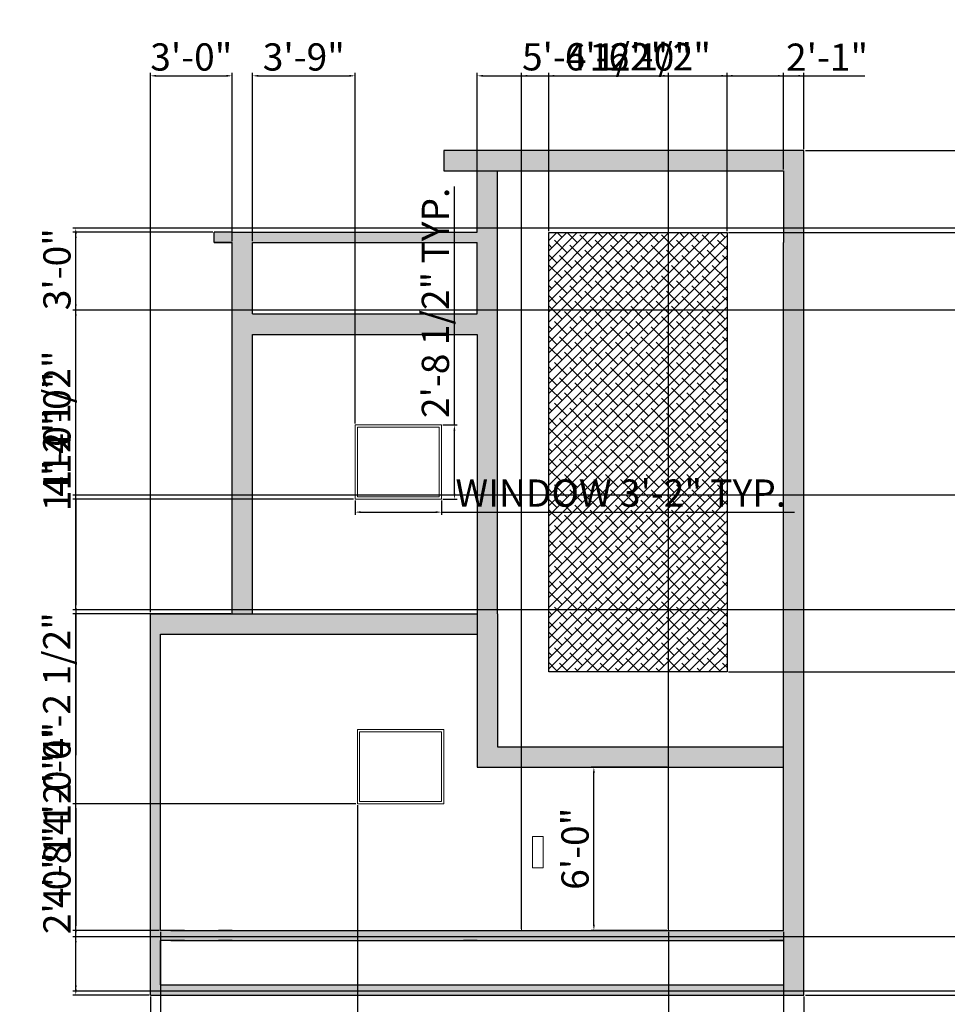
# Model space of a CAD drawing. Units: inches. Extents: x 2693 to 3501, y 1190 to 2292.
# Tile 3 of 4: x 2693 to 3102, y 1858 to 2292. Entities that reach past the tile are written whole.
import ezdxf

# ---------------------------------------------------------------- set-up
doc = ezdxf.new("R2010")
doc.units = ezdxf.units.IN
for name, color, linetype, lineweight in [('A-ANNO-DIMS', 2, 'Continuous', 18), ('A-DOOR', 3, 'Continuous', 18), ('A-ELEV', 7, 'Continuous', 25), ('A-ELEV-PATT', 252, 'Continuous', 13), ('A-GLAZ', 4, 'Continuous', 18), ('A-SECT-PATT', 252, 'Continuous', 13)]:
    doc.layers.add(name, color=color, linetype=linetype, lineweight=lineweight)
doc.styles.get("Standard").update_dxf_attribs({"font": 'arial.ttf'})
doc.dimstyles.new('ISO-25', dxfattribs={"dimtxt": 12, "dimasz": 2.5, "dimexe": 1.25, "dimexo": 0.625, "dimtad": 1, "dimdec": 1, "dimlunit": 3, "dimtxsty": 'Standard', "dimcen": 2.5, "dimadec": 0, "dimazin": 0, "dimtfac": 1, "dimtdec": 1, "dimtmove": 0, "dimatfit": 3, "dimfxl": 1, "dimarcsym": 0})

# ---------------------------------------------------------------- blocks, each defined once
blk = doc.blocks.new('WIN-ELEV-RECT-38')
for points in [[(0, 32.69), (38.06, 32.69), (38.06, 0), (0, 0)], [(1, 31.69), (37.06, 31.69), (37.06, 1), (1, 1)]]:
    blk.add_lwpolyline(points, close=True)
blk = doc.blocks.new('*D15')
at = {"layer": 'A-ANNO-DIMS', "color": 0, "lineweight": -2, "transparency": 16777216}
for p, q in [((2840.85, 2079.8), (2840.85, 2073.46)), ((2878.91, 2079.8), (2878.91, 2073.46)), ((2843.35, 2074.71), (2876.41, 2074.71)), ((2878.91, 2074.71), (3034.51, 2074.71))]:
    blk.add_line(p, q, dxfattribs=at)
at = {"layer": 'A-ANNO-DIMS', "color": 0, "transparency": 16777216}
for points in [[(2843.35, 2075.13), (2843.35, 2074.3), (2840.85, 2074.71)], [(2876.41, 2075.13), (2876.41, 2074.3), (2878.91, 2074.71)]]:
    blk.add_solid(points, dxfattribs=at)
at = {"layer": 'Defpoints', "color": 0, "transparency": 16777216}
for p in [(2840.85, 2080.42), (2878.91, 2080.42), (2878.91, 2074.71)]:
    blk.add_point(p, dxfattribs=at)
at = {"layer": 'A-ANNO-DIMS', "color": 0, "transparency": 16777216, "insert": (2957.96, 2081.55), "char_height": 12, "attachment_point": 5}
blk.add_mtext('WINDOW 3\'-2" TYP.', dxfattribs=at)
blk = doc.blocks.new('*D16')
at = {"layer": 'A-ANNO-DIMS', "color": 0, "lineweight": -2, "transparency": 16777216}
for p, q in [((2884.62, 2113.11), (2884.62, 2218.17)), ((2879.54, 2113.11), (2885.87, 2113.11)), ((2884.62, 2082.92), (2884.62, 2110.61)), ((2879.54, 2080.42), (2885.87, 2080.42))]:
    blk.add_line(p, q, dxfattribs=at)
at = {"layer": 'A-ANNO-DIMS', "color": 0, "transparency": 16777216}
for points in [[(2884.21, 2110.61), (2885.04, 2110.61), (2884.62, 2113.11)], [(2884.21, 2082.92), (2885.04, 2082.92), (2884.62, 2080.42)]]:
    blk.add_solid(points, dxfattribs=at)
at = {"layer": 'Defpoints', "color": 0, "transparency": 16777216}
for p in [(2878.91, 2113.11), (2884.62, 2113.11), (2878.91, 2080.42)]:
    blk.add_point(p, dxfattribs=at)
at = {"layer": 'A-ANNO-DIMS', "color": 0, "transparency": 16777216, "insert": (2877.79, 2166.89), "char_height": 12, "attachment_point": 5, "rotation": 90}
blk.add_mtext('2\'-8 1/2" TYP.', dxfattribs=at)
blk = doc.blocks.new('*D32')
at = {"layer": 'A-ANNO-DIMS', "color": 0, "lineweight": -2, "transparency": 16777216}
for p, q in [((2750.68, 2030.62), (2750.68, 2268.14)), ((2753.18, 2266.89), (2784.18, 2266.89)), ((2786.68, 2194.12), (2786.68, 2268.14))]:
    blk.add_line(p, q, dxfattribs=at)
at = {"layer": 'A-ANNO-DIMS', "color": 0, "transparency": 16777216}
for points in [[(2753.18, 2267.31), (2753.18, 2266.48), (2750.68, 2266.89)], [(2784.18, 2267.31), (2784.18, 2266.48), (2786.68, 2266.89)]]:
    blk.add_solid(points, dxfattribs=at)
at = {"layer": 'Defpoints', "color": 0, "transparency": 16777216}
for p in [(2786.68, 2266.89), (2786.68, 2193.49), (2750.68, 2029.99)]:
    blk.add_point(p, dxfattribs=at)
at = {"layer": 'A-ANNO-DIMS', "color": 0, "transparency": 16777216, "insert": (2768.68, 2273.65), "char_height": 12, "attachment_point": 5}
blk.add_mtext('3\'-0"', dxfattribs=at)
blk = doc.blocks.new('*D33')
at = {"layer": 'A-ANNO-DIMS', "color": 0, "lineweight": -2, "transparency": 16777216}
for p, q in [((2894.68, 2198.62), (2894.68, 2268.14)), ((2897.18, 2266.89), (3036.18, 2266.89)), ((3038.68, 2234.62), (3038.68, 2268.14))]:
    blk.add_line(p, q, dxfattribs=at)
at = {"layer": 'A-ANNO-DIMS', "color": 0, "transparency": 16777216}
for points in [[(2897.18, 2267.31), (2897.18, 2266.48), (2894.68, 2266.89)], [(3036.18, 2267.31), (3036.18, 2266.48), (3038.68, 2266.89)]]:
    blk.add_solid(points, dxfattribs=at)
at = {"layer": 'Defpoints', "color": 0, "transparency": 16777216}
for p in [(3038.68, 2266.89), (3038.68, 2233.99), (2894.68, 2197.99)]:
    blk.add_point(p, dxfattribs=at)
at = {"layer": 'A-ANNO-DIMS', "color": 0, "transparency": 16777216, "insert": (2966.68, 2273.65), "char_height": 12, "attachment_point": 5}
blk.add_mtext('12\'-0"', dxfattribs=at)
blk = doc.blocks.new('*D34')
at = {"layer": 'A-ANNO-DIMS', "color": 0, "lineweight": -2, "transparency": 16777216}
for p, q in [((2750.05, 2029.99), (2716.53, 2029.99)), ((2717.78, 1864.49), (2717.78, 2027.49)), ((2750.05, 1861.99), (2716.53, 1861.99))]:
    blk.add_line(p, q, dxfattribs=at)
at = {"layer": 'A-ANNO-DIMS', "color": 0, "transparency": 16777216}
for points in [[(2717.36, 2027.49), (2718.19, 2027.49), (2717.78, 2029.99)], [(2717.36, 1864.49), (2718.19, 1864.49), (2717.78, 1861.99)]]:
    blk.add_solid(points, dxfattribs=at)
at = {"layer": 'Defpoints', "color": 0, "transparency": 16777216}
for p in [(2717.78, 2029.99), (2750.68, 2029.99), (2750.68, 1861.99)]:
    blk.add_point(p, dxfattribs=at)
at = {"layer": 'A-ANNO-DIMS', "color": 0, "transparency": 16777216, "insert": (2711.02, 1945.99), "char_height": 12, "attachment_point": 5, "rotation": 90}
blk.add_mtext('14\'-0"', dxfattribs=at)
blk = doc.blocks.new('*D35')
at = {"layer": 'A-ANNO-DIMS', "color": 0, "lineweight": -2, "transparency": 16777216}
for p, q in [((2778.13, 2197.99), (2716.53, 2197.99)), ((2717.78, 2032.49), (2717.78, 2195.49)), ((2786.05, 2029.99), (2716.53, 2029.99))]:
    blk.add_line(p, q, dxfattribs=at)
at = {"layer": 'A-ANNO-DIMS', "color": 0, "transparency": 16777216}
for points in [[(2717.36, 2195.49), (2718.19, 2195.49), (2717.78, 2197.99)], [(2717.36, 2032.49), (2718.19, 2032.49), (2717.78, 2029.99)]]:
    blk.add_solid(points, dxfattribs=at)
at = {"layer": 'Defpoints', "color": 0, "transparency": 16777216}
for p in [(2717.78, 2197.99), (2778.76, 2197.99), (2786.68, 2029.99)]:
    blk.add_point(p, dxfattribs=at)
at = {"layer": 'A-ANNO-DIMS', "color": 0, "transparency": 16777216, "insert": (2711.02, 2113.99), "char_height": 12, "attachment_point": 5, "rotation": 90}
blk.add_mtext('14\'-0"', dxfattribs=at)
blk = doc.blocks.new('*D36')
at = {"layer": 'A-ANNO-DIMS', "color": 0, "lineweight": -2, "transparency": 16777216}
for p, q in [((2841.85, 1945.66), (2841.85, 1804.29)), ((2755.18, 1889.87), (2755.18, 1804.29)), ((2757.68, 1805.54), (2839.35, 1805.54))]:
    blk.add_line(p, q, dxfattribs=at)
at = {"layer": 'A-ANNO-DIMS', "color": 0, "transparency": 16777216}
for points in [[(2757.68, 1805.95), (2757.68, 1805.12), (2755.18, 1805.54)], [(2839.35, 1805.95), (2839.35, 1805.12), (2841.85, 1805.54)]]:
    blk.add_solid(points, dxfattribs=at)
at = {"layer": 'Defpoints', "color": 0, "transparency": 16777216}
for p in [(2841.85, 1946.28), (2755.18, 1890.49), (2841.85, 1805.54)]:
    blk.add_point(p, dxfattribs=at)
at = {"layer": 'A-ANNO-DIMS', "color": 0, "transparency": 16777216, "insert": (2798.51, 1812.37), "char_height": 12, "attachment_point": 5}
blk.add_mtext('7\'-2 1/2"', dxfattribs=at)
blk = doc.blocks.new('*D37')
at = {"layer": 'A-ANNO-DIMS', "color": 0, "lineweight": -2, "transparency": 16777216}
for p, q in [((2841.23, 1946.28), (2716.53, 1946.28)), ((2717.78, 1943.78), (2717.78, 1892.99)), ((2754.55, 1890.49), (2716.53, 1890.49))]:
    blk.add_line(p, q, dxfattribs=at)
at = {"layer": 'A-ANNO-DIMS', "color": 0, "transparency": 16777216}
for points in [[(2717.36, 1943.78), (2718.19, 1943.78), (2717.78, 1946.28)], [(2717.36, 1892.99), (2718.19, 1892.99), (2717.78, 1890.49)]]:
    blk.add_solid(points, dxfattribs=at)
at = {"layer": 'Defpoints', "color": 0, "transparency": 16777216}
for p in [(2841.85, 1946.28), (2717.78, 1890.49), (2755.18, 1890.49)]:
    blk.add_point(p, dxfattribs=at)
at = {"layer": 'A-ANNO-DIMS', "color": 0, "transparency": 16777216, "insert": (2711.02, 1918.39), "char_height": 12, "attachment_point": 5, "rotation": 90}
blk.add_mtext('4\'-8"', dxfattribs=at)
blk = doc.blocks.new('*D38')
at = {"layer": 'A-ANNO-DIMS', "color": 0, "lineweight": -2, "transparency": 16777216}
for p, q in [((2717.78, 2080.42), (2717.78, 2144.52)), ((2840.23, 2080.42), (2716.53, 2080.42)), ((2717.78, 2032.49), (2717.78, 2077.92)), ((2786.05, 2029.99), (2716.53, 2029.99))]:
    blk.add_line(p, q, dxfattribs=at)
at = {"layer": 'A-ANNO-DIMS', "color": 0, "transparency": 16777216}
for points in [[(2717.36, 2077.92), (2718.19, 2077.92), (2717.78, 2080.42)], [(2717.36, 2032.49), (2718.19, 2032.49), (2717.78, 2029.99)]]:
    blk.add_solid(points, dxfattribs=at)
at = {"layer": 'Defpoints', "color": 0, "transparency": 16777216}
for p in [(2717.78, 2080.42), (2840.85, 2080.42), (2786.68, 2029.99)]:
    blk.add_point(p, dxfattribs=at)
at = {"layer": 'A-ANNO-DIMS', "color": 0, "transparency": 16777216, "insert": (2710.95, 2113.72), "char_height": 12, "attachment_point": 5, "rotation": 90}
blk.add_mtext('4\'-2 1/2"', dxfattribs=at)
blk = doc.blocks.new('*D39')
at = {"layer": 'A-ANNO-DIMS', "color": 0, "lineweight": -2, "transparency": 16777216}
for p, q in [((2795.68, 2194.12), (2795.68, 2268.14)), ((2798.18, 2266.89), (2838.35, 2266.89)), ((2840.85, 2113.74), (2840.85, 2268.14))]:
    blk.add_line(p, q, dxfattribs=at)
at = {"layer": 'A-ANNO-DIMS', "color": 0, "transparency": 16777216}
for points in [[(2798.18, 2267.31), (2798.18, 2266.48), (2795.68, 2266.89)], [(2838.35, 2267.31), (2838.35, 2266.48), (2840.85, 2266.89)]]:
    blk.add_solid(points, dxfattribs=at)
at = {"layer": 'Defpoints', "color": 0, "transparency": 16777216}
for p in [(2840.85, 2266.89), (2795.68, 2193.49), (2840.85, 2113.11)]:
    blk.add_point(p, dxfattribs=at)
at = {"layer": 'A-ANNO-DIMS', "color": 0, "transparency": 16777216, "insert": (2818.26, 2273.65), "char_height": 12, "attachment_point": 5}
blk.add_mtext('3\'-9"', dxfattribs=at)
blk = doc.blocks.new('*D40')
at = {"layer": 'A-ANNO-DIMS', "color": 0, "lineweight": -2, "transparency": 16777216}
for p, q in [((2914.25, 1891.12), (2914.25, 2268.14)), ((2916.75, 2266.89), (2976.49, 2266.89)), ((2978.99, 1891.12), (2978.99, 2268.14))]:
    blk.add_line(p, q, dxfattribs=at)
at = {"layer": 'A-ANNO-DIMS', "color": 0, "transparency": 16777216}
for points in [[(2916.75, 2267.31), (2916.75, 2266.48), (2914.25, 2266.89)], [(2976.49, 2267.31), (2976.49, 2266.48), (2978.99, 2266.89)]]:
    blk.add_solid(points, dxfattribs=at)
at = {"layer": 'Defpoints', "color": 0, "transparency": 16777216}
for p in [(2978.99, 2266.89), (2914.25, 1890.49), (2978.99, 1890.49)]:
    blk.add_point(p, dxfattribs=at)
at = {"layer": 'A-ANNO-DIMS', "color": 0, "transparency": 16777216, "insert": (2946.62, 2273.72), "char_height": 12, "attachment_point": 5}
blk.add_mtext('5\'-4 1/2"', dxfattribs=at)
blk = doc.blocks.new('*D41')
at = {"layer": 'A-ANNO-DIMS', "color": 0, "lineweight": -2, "transparency": 16777216}
for p, q in [((2978.99, 1889.87), (2978.99, 1804.29)), ((3029.68, 1889.87), (3029.68, 1804.29)), ((2981.49, 1805.54), (3027.18, 1805.54)), ((3029.68, 1805.54), (3093.77, 1805.54))]:
    blk.add_line(p, q, dxfattribs=at)
at = {"layer": 'A-ANNO-DIMS', "color": 0, "transparency": 16777216}
for points in [[(2981.49, 1805.95), (2981.49, 1805.12), (2978.99, 1805.54)], [(3027.18, 1805.95), (3027.18, 1805.12), (3029.68, 1805.54)]]:
    blk.add_solid(points, dxfattribs=at)
at = {"layer": 'Defpoints', "color": 0, "transparency": 16777216}
for p in [(2978.99, 1890.49), (3029.68, 1890.49), (3029.68, 1805.54)]:
    blk.add_point(p, dxfattribs=at)
at = {"layer": 'A-ANNO-DIMS', "color": 0, "transparency": 16777216, "insert": (3062.97, 1812.37), "char_height": 12, "attachment_point": 5}
blk.add_mtext('4\'-2 1/2"', dxfattribs=at)
blk = doc.blocks.new('*D42')
at = {"layer": 'A-ANNO-DIMS', "color": 0, "lineweight": -2, "transparency": 16777216}
for p, q in [((2978.36, 1962.38), (2944.84, 1962.38)), ((2946.09, 1892.99), (2946.09, 1959.88)), ((2978.36, 1890.49), (2944.84, 1890.49))]:
    blk.add_line(p, q, dxfattribs=at)
at = {"layer": 'A-ANNO-DIMS', "color": 0, "transparency": 16777216}
for points in [[(2945.67, 1959.88), (2946.5, 1959.88), (2946.09, 1962.38)], [(2945.67, 1892.99), (2946.5, 1892.99), (2946.09, 1890.49)]]:
    blk.add_solid(points, dxfattribs=at)
at = {"layer": 'Defpoints', "color": 0, "transparency": 16777216}
for p in [(2946.09, 1962.38), (2978.99, 1962.38), (2978.99, 1890.49)]:
    blk.add_point(p, dxfattribs=at)
at = {"layer": 'A-ANNO-DIMS', "color": 0, "transparency": 16777216, "insert": (2939.33, 1926.44), "char_height": 12, "attachment_point": 5, "rotation": 90}
blk.add_mtext('6\'-0"', dxfattribs=at)
blk = doc.blocks.new('*D43')
at = {"layer": 'A-ANNO-DIMS', "color": 0, "lineweight": -2, "transparency": 16777216}
for p, q in [((2926.19, 2198.48), (2926.19, 2268.14)), ((2928.69, 2266.89), (3002.26, 2266.89)), ((3004.76, 2198.48), (3004.76, 2268.14))]:
    blk.add_line(p, q, dxfattribs=at)
at = {"layer": 'A-ANNO-DIMS', "color": 0, "transparency": 16777216}
for points in [[(2928.69, 2267.31), (2928.69, 2266.48), (2926.19, 2266.89)], [(3002.26, 2267.31), (3002.26, 2266.48), (3004.76, 2266.89)]]:
    blk.add_solid(points, dxfattribs=at)
at = {"layer": 'Defpoints', "color": 0, "transparency": 16777216}
for p in [(3004.76, 2266.89), (2926.19, 2197.86), (3004.76, 2197.86)]:
    blk.add_point(p, dxfattribs=at)
at = {"layer": 'A-ANNO-DIMS', "color": 0, "transparency": 16777216, "insert": (2965.47, 2273.72), "char_height": 12, "attachment_point": 5}
blk.add_mtext('6\'-6 1/2"', dxfattribs=at)
blk = doc.blocks.new('*D44')
at = {"layer": 'A-ANNO-DIMS', "color": 0, "lineweight": -2, "transparency": 16777216}
for p, q in [((3004.76, 2198.48), (3004.76, 2268.14)), ((3007.26, 2266.89), (3027.18, 2266.89)), ((3029.68, 2225.62), (3029.68, 2268.14)), ((3029.68, 2266.89), (3065.53, 2266.89))]:
    blk.add_line(p, q, dxfattribs=at)
at = {"layer": 'A-ANNO-DIMS', "color": 0, "transparency": 16777216}
for points in [[(3007.26, 2267.31), (3007.26, 2266.48), (3004.76, 2266.89)], [(3027.18, 2267.31), (3027.18, 2266.48), (3029.68, 2266.89)]]:
    blk.add_solid(points, dxfattribs=at)
at = {"layer": 'Defpoints', "color": 0, "transparency": 16777216}
for p in [(3029.68, 2266.89), (3029.68, 2224.99), (3004.76, 2197.86)]:
    blk.add_point(p, dxfattribs=at)
at = {"layer": 'A-ANNO-DIMS', "color": 0, "transparency": 16777216, "insert": (3048.85, 2273.54), "char_height": 12, "attachment_point": 5}
blk.add_mtext('2\'-1"', dxfattribs=at)
blk = doc.blocks.new('*D45')
at = {"layer": 'A-ANNO-DIMS', "color": 0, "lineweight": -2, "transparency": 16777216}
for p, q in [((3005.39, 2197.86), (3435.42, 2197.86)), ((3434.17, 2006.84), (3434.17, 2195.36)), ((3005.39, 2004.34), (3435.42, 2004.34))]:
    blk.add_line(p, q, dxfattribs=at)
at = {"layer": 'A-ANNO-DIMS', "color": 0, "transparency": 16777216}
for points in [[(3433.76, 2195.36), (3434.59, 2195.36), (3434.17, 2197.86)], [(3433.76, 2006.84), (3434.59, 2006.84), (3434.17, 2004.34)]]:
    blk.add_solid(points, dxfattribs=at)
at = {"layer": 'Defpoints', "color": 0, "transparency": 16777216}
for p in [(3004.76, 2197.86), (3434.17, 2197.86), (3004.76, 2004.34)]:
    blk.add_point(p, dxfattribs=at)
at = {"layer": 'A-ANNO-DIMS', "color": 0, "transparency": 16777216, "insert": (3427.34, 2101.1), "char_height": 12, "attachment_point": 5, "rotation": 90}
blk.add_mtext('16\'-1 1/2"', dxfattribs=at)
blk = doc.blocks.new('*D46')
at = {"layer": 'A-ANNO-DIMS', "color": 0, "lineweight": -2, "transparency": 16777216}
for p, q in [((2750.68, 1861.37), (2750.68, 1804.29)), ((3038.68, 1861.37), (3038.68, 1804.29)), ((2753.18, 1805.54), (3036.18, 1805.54))]:
    blk.add_line(p, q, dxfattribs=at)
at = {"layer": 'A-ANNO-DIMS', "color": 0, "transparency": 16777216}
for points in [[(2753.18, 1805.95), (2753.18, 1805.12), (2750.68, 1805.54)], [(3036.18, 1805.95), (3036.18, 1805.12), (3038.68, 1805.54)]]:
    blk.add_solid(points, dxfattribs=at)
at = {"layer": 'Defpoints', "color": 0, "transparency": 16777216}
for p in [(2750.68, 1861.99), (3038.68, 1861.99), (3038.68, 1805.54)]:
    blk.add_point(p, dxfattribs=at)
at = {"layer": 'A-ANNO-DIMS', "color": 0, "transparency": 16777216, "insert": (2894.68, 1812.29), "char_height": 12, "attachment_point": 5}
blk.add_mtext('24\'-0"', dxfattribs=at)
blk = doc.blocks.new('*D47')
at = {"layer": 'A-ANNO-DIMS', "color": 0, "lineweight": -2, "transparency": 16777216}
for p, q in [((3039.3, 2233.99), (3435.42, 2233.99)), ((3434.17, 1864.49), (3434.17, 2231.49)), ((3039.3, 1861.99), (3435.42, 1861.99))]:
    blk.add_line(p, q, dxfattribs=at)
at = {"layer": 'A-ANNO-DIMS', "color": 0, "transparency": 16777216}
for points in [[(3433.76, 2231.49), (3434.59, 2231.49), (3434.17, 2233.99)], [(3433.76, 1864.49), (3434.59, 1864.49), (3434.17, 1861.99)]]:
    blk.add_solid(points, dxfattribs=at)
at = {"layer": 'Defpoints', "color": 0, "transparency": 16777216}
for p in [(3038.68, 2233.99), (3434.17, 2233.99), (3038.68, 1861.99)]:
    blk.add_point(p, dxfattribs=at)
at = {"layer": 'A-ANNO-DIMS', "color": 0, "transparency": 16777216, "insert": (3427.42, 2047.99), "char_height": 12, "attachment_point": 5, "rotation": 90}
blk.add_mtext('31\'-0"', dxfattribs=at)
blk = doc.blocks.new('*D48')
at = {"layer": 'A-ANNO-DIMS', "color": 0, "lineweight": -2, "transparency": 16777216}
for p, q in [((2717.78, 1887.72), (2717.78, 1923.57)), ((3115.65, 1887.72), (2716.53, 1887.72)), ((2717.78, 1866.22), (2717.78, 1885.22)), ((3112.65, 1863.72), (2716.53, 1863.72))]:
    blk.add_line(p, q, dxfattribs=at)
at = {"layer": 'A-ANNO-DIMS', "color": 0, "transparency": 16777216}
for points in [[(2717.36, 1885.22), (2718.19, 1885.22), (2717.78, 1887.72)], [(2717.36, 1866.22), (2718.19, 1866.22), (2717.78, 1863.72)]]:
    blk.add_solid(points, dxfattribs=at)
at = {"layer": 'Defpoints', "color": 0, "transparency": 16777216}
for p in [(2717.78, 1887.72), (3116.27, 1887.72), (3113.27, 1863.72)]:
    blk.add_point(p, dxfattribs=at)
at = {"layer": 'A-ANNO-DIMS', "color": 0, "transparency": 16777216, "insert": (2711.02, 1906.89), "char_height": 12, "attachment_point": 5, "rotation": 90}
blk.add_mtext('2\'-0"', dxfattribs=at)
blk = doc.blocks.new('*D49')
at = {"layer": 'A-ANNO-DIMS', "color": 0, "lineweight": -2, "transparency": 16777216}
for p, q in [((3112.65, 2031.72), (2716.53, 2031.72)), ((2717.78, 1890.22), (2717.78, 2029.22)), ((3121.65, 1887.72), (2716.53, 1887.72))]:
    blk.add_line(p, q, dxfattribs=at)
at = {"layer": 'A-ANNO-DIMS', "color": 0, "transparency": 16777216}
for points in [[(2717.36, 2029.22), (2718.19, 2029.22), (2717.78, 2031.72)], [(2717.36, 1890.22), (2718.19, 1890.22), (2717.78, 1887.72)]]:
    blk.add_solid(points, dxfattribs=at)
at = {"layer": 'Defpoints', "color": 0, "transparency": 16777216}
for p in [(2717.78, 2031.72), (3113.27, 2031.72), (3122.27, 1887.72)]:
    blk.add_point(p, dxfattribs=at)
at = {"layer": 'A-ANNO-DIMS', "color": 0, "transparency": 16777216, "insert": (2711.02, 1959.72), "char_height": 12, "attachment_point": 5, "rotation": 90}
blk.add_mtext('12\'-0"', dxfattribs=at)
blk = doc.blocks.new('*D50')
at = {"layer": 'A-ANNO-DIMS', "color": 0, "lineweight": -2, "transparency": 16777216}
for p, q in [((3157.65, 2163.72), (2716.53, 2163.72)), ((2717.78, 2034.22), (2717.78, 2161.22)), ((3112.65, 2031.72), (2716.53, 2031.72))]:
    blk.add_line(p, q, dxfattribs=at)
at = {"layer": 'A-ANNO-DIMS', "color": 0, "transparency": 16777216}
for points in [[(2717.36, 2161.22), (2718.19, 2161.22), (2717.78, 2163.72)], [(2717.36, 2034.22), (2718.19, 2034.22), (2717.78, 2031.72)]]:
    blk.add_solid(points, dxfattribs=at)
at = {"layer": 'Defpoints', "color": 0, "transparency": 16777216}
for p in [(2717.78, 2163.72), (3158.27, 2163.72), (3113.27, 2031.72)]:
    blk.add_point(p, dxfattribs=at)
at = {"layer": 'A-ANNO-DIMS', "color": 0, "transparency": 16777216, "insert": (2711.02, 2097.72), "char_height": 12, "attachment_point": 5, "rotation": 90}
blk.add_mtext('11\'-0"', dxfattribs=at)
blk = doc.blocks.new('*D51')
at = {"layer": 'A-ANNO-DIMS', "color": 0, "lineweight": -2, "transparency": 16777216}
for p, q in [((3148.65, 2199.72), (2716.53, 2199.72)), ((2717.78, 2166.22), (2717.78, 2197.22)), ((3157.65, 2163.72), (2716.53, 2163.72))]:
    blk.add_line(p, q, dxfattribs=at)
at = {"layer": 'A-ANNO-DIMS', "color": 0, "transparency": 16777216}
for points in [[(2717.36, 2197.22), (2718.19, 2197.22), (2717.78, 2199.72)], [(2717.36, 2166.22), (2718.19, 2166.22), (2717.78, 2163.72)]]:
    blk.add_solid(points, dxfattribs=at)
at = {"layer": 'Defpoints', "color": 0, "transparency": 16777216}
for p in [(2717.78, 2199.72), (3149.27, 2199.72), (3158.27, 2163.72)]:
    blk.add_point(p, dxfattribs=at)
at = {"layer": 'A-ANNO-DIMS', "color": 0, "transparency": 16777216, "insert": (2711.02, 2181.72), "char_height": 12, "attachment_point": 5, "rotation": 90}
blk.add_mtext('3\'-0"', dxfattribs=at)
blk = doc.blocks.new('*D56')
at = {"layer": 'A-ANNO-DIMS', "color": 0, "lineweight": -2, "transparency": 16777216}
for p, q in [((3202.82, 2082.15), (2716.53, 2082.15)), ((2717.78, 2079.65), (2717.78, 2034.22)), ((3157.65, 2031.72), (2716.53, 2031.72)), ((2717.78, 2031.72), (2717.78, 1967.62))]:
    blk.add_line(p, q, dxfattribs=at)
at = {"layer": 'A-ANNO-DIMS', "color": 0, "transparency": 16777216}
for points in [[(2717.36, 2079.65), (2718.19, 2079.65), (2717.78, 2082.15)], [(2717.36, 2034.22), (2718.19, 2034.22), (2717.78, 2031.72)]]:
    blk.add_solid(points, dxfattribs=at)
at = {"layer": 'Defpoints', "color": 0, "transparency": 16777216}
for p in [(3203.45, 2082.15), (2717.78, 2031.72), (3158.27, 2031.72)]:
    blk.add_point(p, dxfattribs=at)
at = {"layer": 'A-ANNO-DIMS', "color": 0, "transparency": 16777216, "insert": (2710.95, 1998.42), "char_height": 12, "attachment_point": 5, "rotation": 90}
blk.add_mtext('4\'-2 1/2"', dxfattribs=at)

msp = doc.modelspace()

# ---------------------------------------------------------------- hatches: boundary and pattern name
at = {"layer": 'A-ELEV-PATT'}
h = msp.add_hatch(dxfattribs=at)
h.set_pattern_fill('ANSI38', color=256)
h.paths.add_polyline_path([(3004.76, 2197.86), (2926.19, 2197.86), (2926.19, 2004.34), (3004.76, 2004.34)])
at = {"layer": 'A-SECT-PATT'}
h = msp.add_hatch(color=256, dxfattribs=at)
h.dxf.hatch_style = 1
h.paths.add_polyline_path([(3038.68, 2197.99), (3038.68, 2233.99), (2879.9, 2233.99), (2879.9, 2224.99), (3029.68, 2224.99), (3029.68, 2193.49), (3029.68, 2161.99), (3029.68, 2029.99), (3029.68, 1962.38), (3029.68, 1890.49), (2903.68, 1890.49), (2786.68, 1890.49), (2780.68, 1890.49), (2759.68, 1890.49), (2755.18, 1890.49), (2755.18, 2020.99), (2894.68, 2020.99), (2894.68, 2029.99), (2786.68, 2029.99), (2750.68, 2029.99), (2750.68, 1861.99), (3038.68, 1861.99), (3038.68, 1885.99)])
h.paths.add_polyline_path([(3029.68, 1885.99), (3029.68, 1866.49), (2755.18, 1866.49), (2755.18, 1885.99), (2759.68, 1885.99), (2765.68, 1885.99), (2786.68, 1885.99), (2903.68, 1885.99), (2909.68, 1885.99), (2912.68, 1885.99)], flags=16)
h.paths.add_polyline_path([(2903.68, 2152.99), (2903.68, 2224.99), (2894.68, 2224.99), (2894.68, 2197.99), (2894.43, 2197.99), (2786.68, 2197.99), (2778.76, 2197.99), (2778.76, 2193.49), (2786.68, 2193.49), (2786.68, 2029.99), (2795.68, 2029.99), (2795.68, 2152.99), (2894.68, 2152.99), (2894.68, 2029.99), (2894.68, 1971.38), (2894.68, 1962.38), (3029.68, 1962.38), (3029.68, 1971.38), (2903.68, 1971.38), (2903.68, 2029.99)], flags=17)
h.paths.add_polyline_path([(2894.68, 2161.99), (2795.68, 2161.99), (2795.68, 2193.49), (2894.68, 2193.49)], flags=16)
h.paths.add_polyline_path([(3401.27, 2199.72), (3149.27, 2199.72), (3149.27, 2031.72), (3113.27, 2031.72), (3113.27, 1863.72), (3116.27, 1863.72), (3116.27, 1887.72), (3122.27, 1887.72), (3122.27, 2022.72), (3149.27, 2022.72), (3149.27, 1887.72), (3143.27, 1887.72), (3143.27, 1863.72), (3164.27, 1863.72), (3164.27, 1887.72), (3158.27, 1887.72), (3158.27, 2022.72), (3257.27, 2022.72), (3257.27, 1887.72), (3251.27, 1887.72), (3251.27, 1863.72), (3272.27, 1863.72), (3272.27, 1887.72), (3266.27, 1887.72), (3266.27, 2022.72), (3392.27, 2022.72), (3392.27, 1887.72), (3398.27, 1887.72), (3398.27, 1863.72), (3401.27, 1863.72), (3401.27, 1887.72)])
h.paths.add_polyline_path([(3257.27, 2031.72), (3158.27, 2031.72), (3158.27, 2195.22), (3392.27, 2195.22), (3392.27, 2163.72), (3158.27, 2163.72), (3158.27, 2154.72), (3257.27, 2154.72)], flags=16)
h.paths.add_polyline_path([(3266.27, 2031.72), (3266.27, 2154.72), (3392.27, 2154.72), (3392.27, 2031.72)], flags=16)
h.paths.add_polyline_path([(3266.27, 2082.15), (3266.27, 2114.83), (3317.96, 2114.83), (3317.96, 2082.15)], flags=0)
h.paths.add_polyline_path([(3241.51, 2082.15), (3203.45, 2082.15), (3203.45, 2114.83), (3241.51, 2114.83)], flags=0)
h.paths.add_polyline_path([(3240.51, 2083.15), (3204.45, 2083.15), (3204.45, 2113.83), (3240.51, 2113.83)], flags=0)
h.paths.add_polyline_path([(3329.27, 2031.72), (3329.27, 2114.83), (3355.99, 2114.83), (3355.99, 2031.72)], flags=0)

# ---------------------------------------------------------------- linework, layer by layer
at = {"layer": 'A-DOOR'}
for p, q in [((2914.25, 1890.49), (2914.25, 1962.38)), ((2978.99, 1890.49), (2978.99, 1962.38))]:
    msp.add_line(p, q, dxfattribs=at)
msp.add_lwpolyline([(2923.73, 1931.83), (2919.05, 1931.83), (2919.05, 1918.03), (2923.73, 1918.03)], close=True, dxfattribs=at)
at = {"layer": 'A-ELEV'}
for p, q in [((3038.68, 2233.99), (2879.9, 2233.99)), ((2879.9, 2233.99), (2879.9, 2224.99)), ((3038.68, 2197.99), (3038.68, 2233.99)), ((2879.9, 2224.99), (3029.68, 2224.99)), ((2879.9, 2224.99), (2879.9, 2224.99)), ((2894.68, 2197.99), (2894.68, 2224.99)), ((2903.68, 2152.99), (2903.68, 2224.99)), ((3029.68, 2224.99), (3029.68, 2193.49)), ((2786.68, 2197.99), (2778.76, 2197.99)), ((2778.76, 2193.49), (2778.76, 2197.99)), ((2786.68, 2197.99), (2894.68, 2197.99)), ((2894.68, 2197.99), (2894.43, 2197.99)), ((3038.68, 1885.99), (3038.68, 2197.99)), ((2778.76, 2193.49), (2786.68, 2193.49)), ((2786.68, 2193.49), (2778.76, 2193.49)), ((2786.68, 2029.99), (2786.68, 2193.49)), ((2795.68, 2193.49), (2894.68, 2193.49)), ((2795.68, 2161.99), (2795.68, 2193.49)), ((2894.68, 2161.99), (2894.68, 2193.49)), ((3029.68, 2029.99), (3029.68, 2193.49)), ((3029.68, 2161.99), (3029.68, 2193.49)), ((2786.68, 2152.99), (2786.68, 2161.99)), ((2795.68, 2161.99), (2894.68, 2161.99)), ((2795.68, 2152.99), (2894.68, 2152.99)), ((2795.68, 2029.99), (2795.68, 2152.99)), ((2894.68, 2152.99), (2894.68, 2029.99)), ((2903.68, 2029.99), (2903.68, 2152.99)), ((2750.68, 2029.99), (2786.68, 2029.99)), ((2750.68, 1861.99), (2750.68, 2029.99)), ((2786.68, 2029.99), (2894.68, 2029.99)), ((2894.68, 2029.99), (2894.68, 1971.38)), ((2903.68, 2029.99), (2903.68, 1971.38)), ((3029.68, 1962.38), (3029.68, 2029.99)), ((2755.18, 2020.99), (2894.68, 2020.99)), ((2755.18, 1890.49), (2755.18, 2020.99)), ((2759.68, 2020.99), (2786.68, 2020.99)), ((3029.68, 1890.49), (3029.68, 2020.99)), ((2894.68, 1971.38), (2894.68, 1962.38)), ((2903.68, 1971.38), (3029.68, 1971.38)), ((2894.68, 1962.38), (3029.68, 1962.38)), ((2759.68, 1890.49), (2755.18, 1890.49)), ((2765.68, 1890.49), (2759.68, 1890.49)), ((2759.68, 1890.49), (2786.68, 1890.49)), ((2786.68, 1890.49), (2780.68, 1890.49)), ((2786.68, 1890.49), (2903.68, 1890.49)), ((2903.68, 1890.49), (3029.68, 1890.49)), ((2759.68, 1885.99), (2755.18, 1885.99)), ((2755.18, 1866.49), (2755.18, 1885.99)), ((2759.68, 1885.99), (2786.68, 1885.99)), ((2759.68, 1885.99), (2765.68, 1885.99)), ((2765.68, 1885.99), (2759.68, 1885.99)), ((2786.68, 1885.99), (2780.68, 1885.99)), ((2786.68, 1885.99), (2903.68, 1885.99)), ((2795.68, 1885.99), (2801.68, 1885.99)), ((2894.68, 1885.99), (2888.68, 1885.99)), ((2903.68, 1885.99), (3029.68, 1885.99)), ((2903.68, 1885.99), (2912.68, 1885.99)), ((2903.68, 1885.99), (2909.68, 1885.99)), ((3029.68, 1885.99), (3023.68, 1885.99)), ((3029.68, 1885.99), (3029.68, 1866.49)), ((3038.68, 1861.99), (3038.68, 1885.99)), ((2755.18, 1866.49), (3029.68, 1866.49)), ((2750.68, 1861.99), (3038.68, 1861.99))]:
    msp.add_line(p, q, dxfattribs=at)
msp.add_lwpolyline([(2926.19, 2197.86), (3004.76, 2197.86), (3004.76, 2004.34), (2926.19, 2004.34)], close=True, dxfattribs=at)
msp.add_lwpolyline([(2966.68, 1885.99), (2993.4, 1885.99)], dxfattribs=at)

# ---------------------------------------------------------------- block references
at = {"layer": 'A-GLAZ'}
for p in [(2840.85, 2080.42), (2841.85, 1946.28)]:
    msp.add_blockref('WIN-ELEV-RECT-38', p, dxfattribs=at)

# ---------------------------------------------------------------- dimensions: what is measured, and where the dimension line sits
at = {"layer": 'A-ANNO-DIMS'}
for base, p1, p2, picture, middle in [((2978.99, 2266.89), (2914.25, 1890.49), (2978.99, 1890.49), '*D40', (2946.62, 2273.72)), ((3004.76, 2266.89), (2926.19, 2197.86), (3004.76, 2197.86), '*D43', (2965.47, 2273.72)), ((2786.68, 2266.89), (2750.68, 2029.99), (2786.68, 2193.49), '*D32', (2768.68, 2273.65)), ((2840.85, 2266.89), (2795.68, 2193.49), (2840.85, 2113.11), '*D39', (2818.26, 2273.65)), ((3038.68, 2266.89), (2894.68, 2197.99), (3038.68, 2233.99), '*D33', (2966.68, 2273.65)), ((3029.68, 2266.89), (3004.76, 2197.86), (3029.68, 2224.99), '*D44', (3048.85, 2273.54)), ((2841.85, 1805.54), (2755.18, 1890.49), (2841.85, 1946.28), '*D36', (2798.51, 1812.37)), ((3029.68, 1805.54), (2978.99, 1890.49), (3029.68, 1890.49), '*D41', (3062.97, 1812.37)), ((3038.68, 1805.54), (2750.68, 1861.99), (3038.68, 1861.99), '*D46', (2894.68, 1812.29))]:
    dim = msp.add_linear_dim(base=base, p1=p1, p2=p2, dimstyle='ISO-25', override={"dimdec": 1, "dimlfac": 1, "dimrnd": 0, "dimzin": 1, "dimdsep": 46, "dimlunit": 4, "dimfrac": 2}, dxfattribs=at)
    dim.commit()
    dim.dimension.update_dxf_attribs({"geometry": picture, "text_midpoint": middle})
for base, p1, p2, picture, middle in [((3434.17, 2233.99), (3038.68, 1861.99), (3038.68, 2233.99), '*D47', (3427.42, 2047.99)), ((2717.78, 2199.72), (3158.27, 2163.72), (3149.27, 2199.72), '*D51', (2711.02, 2181.72)), ((2717.78, 2197.99), (2786.68, 2029.99), (2778.76, 2197.99), '*D35', (2711.02, 2113.99)), ((3434.17, 2197.86), (3004.76, 2004.34), (3004.76, 2197.86), '*D45', (3427.34, 2101.1)), ((2717.78, 2163.72), (3113.27, 2031.72), (3158.27, 2163.72), '*D50', (2711.02, 2097.72)), ((2717.78, 2080.42), (2786.68, 2029.99), (2840.85, 2080.42), '*D38', (2710.95, 2113.72)), ((2717.78, 2031.72), (3203.45, 2082.15), (3158.27, 2031.72), '*D56', (2710.95, 1998.42)), ((2717.78, 2031.72), (3122.27, 1887.72), (3113.27, 2031.72), '*D49', (2711.02, 1959.72)), ((2717.78, 2029.99), (2750.68, 1861.99), (2750.68, 2029.99), '*D34', (2711.02, 1945.99)), ((2946.09, 1962.38), (2978.99, 1890.49), (2978.99, 1962.38), '*D42', (2939.33, 1926.44)), ((2717.78, 1890.49), (2841.85, 1946.28), (2755.18, 1890.49), '*D37', (2711.02, 1918.39)), ((2717.78, 1887.72), (3113.27, 1863.72), (3116.27, 1887.72), '*D48', (2711.02, 1906.89))]:
    dim = msp.add_linear_dim(base=base, p1=p1, p2=p2, angle=90, dimstyle='ISO-25', override={"dimdec": 1, "dimlfac": 1, "dimrnd": 0, "dimzin": 1, "dimdsep": 46, "dimlunit": 4, "dimfrac": 2}, dxfattribs=at)
    dim.commit()
    dim.dimension.update_dxf_attribs({"geometry": picture, "text_midpoint": middle})
dim = msp.add_linear_dim(base=(2884.62, 2113.11), p1=(2878.91, 2080.42), p2=(2878.91, 2113.11), angle=90, text='<> TYP.', dimstyle='ISO-25', override={"dimdec": 1, "dimlfac": 1, "dimrnd": 0, "dimzin": 1, "dimdsep": 46, "dimlunit": 4, "dimfrac": 2}, dxfattribs=at)
dim.commit()
dim.dimension.update_dxf_attribs({"geometry": '*D16', "text_midpoint": (2877.79, 2166.89)})
dim = msp.add_linear_dim(base=(2878.91, 2074.71), p1=(2840.85, 2080.42), p2=(2878.91, 2080.42), text='WINDOW <> TYP.', dimstyle='ISO-25', override={"dimdec": 1, "dimlfac": 1, "dimrnd": 0, "dimzin": 1, "dimdsep": 46, "dimlunit": 4, "dimfrac": 2}, dxfattribs=at)
dim.commit()
dim.dimension.update_dxf_attribs({"geometry": '*D15', "text_midpoint": (2957.96, 2081.55)})

doc.saveas('drawing.dxf')
